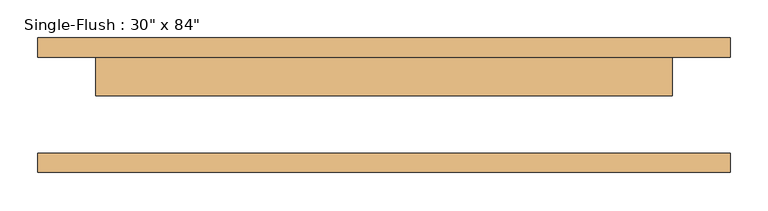
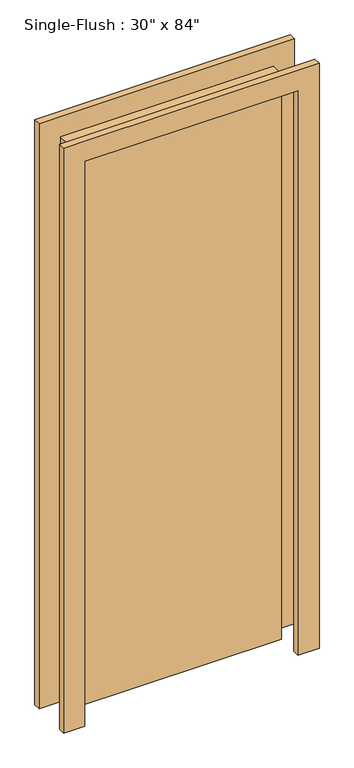
"""IFC4 building model written with IfcOpenShell, lengths in millimetres: door geometry."""

from ifc_helpers import new_model, si_unit, frame, origin, origin_with_axes, place, context, project, spatial, polyline, outline, extrude, source, transform, mapped, element, save


def door_4d6c7550(model_context):
    return source(origin(), model_context, "Body", "SweptSolid", [
        extrude(outline(polyline([(2209.8, -457.2), (0.0, -457.2), (0.0, -381.0), (2133.6, -381.0), (2133.6, 381.0), (0.0, 381.0), (0.0, 457.2), (2209.8, 457.2), (2209.8, -457.2)])), frame((0.0, 63.5, 0.0), z_axis=(0.0, 1.0, 0.0), x_axis=(0.0, 0.0, 1.0)), (0.0, 0.0, 1.0), 25.4),
        extrude(outline(polyline([(2209.8, 457.2), (2209.8, -457.2), (0.0, -457.2), (0.0, -381.0), (2133.6, -381.0), (2133.6, 381.0), (0.0, 381.0), (0.0, 457.2), (2209.8, 457.2)])), frame((0.0, -88.9, 0.0), z_axis=(0.0, 1.0, 0.0), x_axis=(0.0, 0.0, 1.0)), (0.0, 0.0, 1.0), 25.4),
        extrude(outline(polyline([(381.0, 12.7), (-381.0, 12.7), (-381.0, 63.5), (381.0, 63.5), (381.0, 12.7)])), origin_with_axes(), (0.0, 0.0, 1.0), 2133.6),
    ])


if __name__ == "__main__":
    model = new_model("IFC4")
    model_context = context("Model", 3, world=origin())
    ifc_project = project(units=[si_unit("LENGTHUNIT", "METRE", prefix="MILLI")], contexts=[model_context])
    site = spatial("IfcSite", under=ifc_project)
    building = spatial("IfcBuilding", under=site)
    placement = place(None, origin())
    door_shape = door_4d6c7550(model_context)
    element("IfcDoor", 1, ObjectType="Single-Flush : 30\" x 84\"", at=placement, inside=building, context=model_context, shape_type="MappedRepresentation", body=[
        mapped(door_shape, transform((0.0, 0.0, 0.0), x_axis=(1.0, 0.0, 0.0), y_axis=(0.0, 1.0, 0.0), z_axis=(0.0, 0.0, 1.0))),
    ])
    save(model, "model.ifc")

# Revit data of these elements
# Type "Single-Flush : 30\" x 84\""
#   Type Mark = "4"
#   Construction Type Id = "MDOOR"
#   Assembly Code = "C1020"
#   Analytic Construction = "Metal"
#   Thickness = 0' - 2"
#   Heat Transfer Coefficient (U) = 0.651978 BTU/(h·ft²·°F)
#   Height = 7' - 0"
#   Trim Projection Ext = 0' - 1"
#   Trim Projection Int = 0' - 1"
#   Trim Width = 0' - 3"
#   Width = 2' - 6"
#   Define Thermal Properties by = 1
#   Define Thermal Properties by = 1
#   Door Material = Door - Panel
#   Frame Material = Door - Frame
#   Visual Light Transmittance = 0
#   Solar Heat Gain Coefficient = 0
#   Function = (empty or 0)
#   Wall Closure = (empty or 0)
# Element 1 (IfcDoor, "Single-Flush : 30\" x 84\"")
#   Materials on its faces: "Door - Frame", "Door - Panel"
# Materials
#   "Door - Panel": class "Wood", colour RGB 210 159 95, transparency 0, Cost = 0
#   "Door - Frame": colour RGB 118 70 51, transparency 0, Cost = 0
